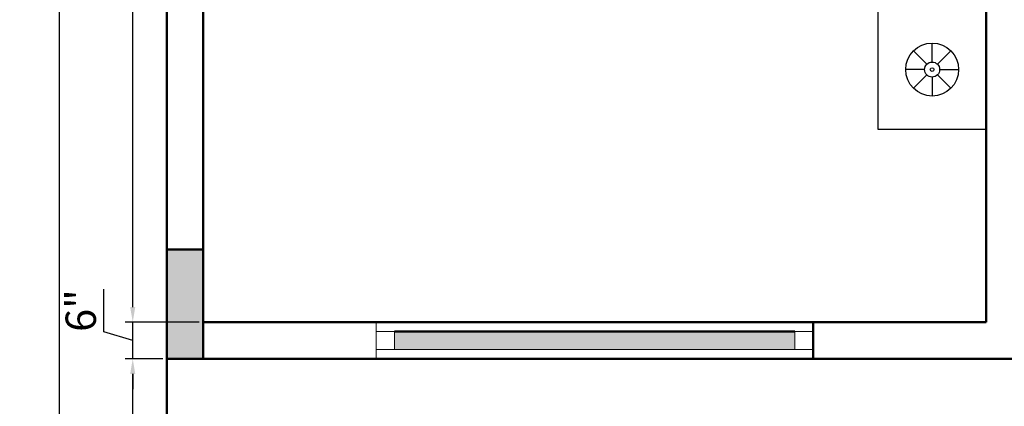
# Model space of a CAD drawing. Units: inches. Extents: x 3064 to 19385, y 846 to 15425.
# Tile 36 of 108: x 5167 to 5329, y 964 to 1028. Entities that reach past the tile are written whole.
import ezdxf

# ---------------------------------------------------------------- set-up
doc = ezdxf.new("R2010")
doc.units = ezdxf.units.IN
for name, color, linetype, lineweight in [('A-ANNO-DIMS', 2, 'Continuous', 18), ('A-COLS', 1, 'Continuous', 35), ('A-FLOR-FIXT', 9, 'Continuous', 18), ('A-GLAZ', 4, 'Continuous', 18), ('A-WALL', 7, 'Continuous', 50)]:
    doc.layers.add(name, color=color, linetype=linetype, lineweight=lineweight)
doc.layers.add('BLOCK', color=6, linetype='Continuous')
doc.styles.get("Standard").update_dxf_attribs({"font": 'arial.ttf'})
doc.dimstyles.new('ISO-25', dxfattribs={"dimtxt": 9, "dimasz": 2.5, "dimexe": 1.25, "dimexo": 0.625, "dimtad": 1, "dimdec": 1, "dimlunit": 3, "dimtxsty": 'Standard', "dimcen": 2.5, "dimadec": 0, "dimazin": 0, "dimtfac": 1, "dimtdec": 1, "dimtmove": 0, "dimatfit": 3, "dimfxl": 1, "dimarcsym": 0})

# ---------------------------------------------------------------- blocks, each defined once
blk = doc.blocks.new('A$C52E67D0D')
at = {"layer": 'BLOCK'}
for p, q in [((2229.3, 1596.3), (2173.3, 1652.3)), ((2251.5, 1605.5), (2251.5, 1684.7)), ((2273.7, 1596.3), (2329.7, 1652.3)), ((2220.1, 1574.1), (2140.9, 1574.1)), ((2282.9, 1574.1), (2362.1, 1574.1)), ((2229.3, 1551.9), (2173.3, 1495.9)), ((2251.5, 1542.8), (2251.5, 1463.5)), ((2273.7, 1551.9), (2329.7, 1495.9))]:
    blk.add_line(p, q, dxfattribs=at)
blk.add_lwpolyline([(2001, 1348.6), (2001, 1799.6), (2502, 1799.6), (2502, 1348.6)], close=True, dxfattribs=at)
for radius in [110.6, 31.4, 7.46]:
    blk.add_circle((2251.5, 1574.1), radius, dxfattribs=at)
blk = doc.blocks.new('*D68')
at = {"layer": 'A-ANNO-DIMS', "color": 0, "lineweight": -2, "transparency": 16777216}
for p, q in [((5190.39, 972.1), (5184.17, 972.1)), ((5185.42, 902.6), (5185.42, 969.6)), ((5190.39, 900.1), (5184.17, 900.1))]:
    blk.add_line(p, q, dxfattribs=at)
at = {"layer": 'A-ANNO-DIMS', "color": 0, "transparency": 16777216}
for points in [[(5185, 969.6), (5185.83, 969.6), (5185.42, 972.1)], [(5185, 902.6), (5185.83, 902.6), (5185.42, 900.1)]]:
    blk.add_solid(points, dxfattribs=at)
at = {"layer": 'Defpoints', "color": 0, "transparency": 16777216}
for p in [(5185.42, 972.1), (5191.02, 972.1), (5191.02, 900.1)]:
    blk.add_point(p, dxfattribs=at)
at = {"layer": 'A-ANNO-DIMS', "color": 0, "transparency": 16777216, "insert": (5182.24, 936.1), "char_height": 5, "attachment_point": 5, "rotation": 90}
blk.add_mtext("6'", dxfattribs=at)
blk = doc.blocks.new('*D69')
at = {"layer": 'A-ANNO-DIMS', "color": 0, "lineweight": -2, "transparency": 16777216}
for p, q in [((5180.68, 976.52), (5180.68, 983.54)), ((5185.42, 980.6), (5185.42, 983.1)), ((5196.39, 978.1), (5184.17, 978.1)), ((5185.42, 972.1), (5185.42, 978.1)), ((5185.42, 972.1), (5185.42, 978.1)), ((5185.42, 975.1), (5180.68, 976.52)), ((5190.39, 972.1), (5184.17, 972.1)), ((5185.42, 969.6), (5185.42, 967.1))]:
    blk.add_line(p, q, dxfattribs=at)
at = {"layer": 'A-ANNO-DIMS', "color": 0, "transparency": 16777216}
for points in [[(5185, 980.6), (5185.83, 980.6), (5185.42, 978.1)], [(5185, 969.6), (5185.83, 969.6), (5185.42, 972.1)]]:
    blk.add_solid(points, dxfattribs=at)
at = {"layer": 'Defpoints', "color": 0, "transparency": 16777216}
for p in [(5185.42, 978.1), (5197.02, 978.1), (5191.02, 972.1)]:
    blk.add_point(p, dxfattribs=at)
at = {"layer": 'A-ANNO-DIMS', "color": 0, "transparency": 16777216, "insert": (5177.5, 980.03), "char_height": 5, "attachment_point": 5, "rotation": 90}
blk.add_mtext('6"', dxfattribs=at)
blk = doc.blocks.new('*D70')
at = {"layer": 'A-ANNO-DIMS', "color": 0, "lineweight": -2, "transparency": 16777216}
for p, q in [((5196.39, 1176.1), (5184.17, 1176.1)), ((5185.42, 980.6), (5185.42, 1173.6)), ((5196.39, 978.1), (5184.17, 978.1))]:
    blk.add_line(p, q, dxfattribs=at)
at = {"layer": 'A-ANNO-DIMS', "color": 0, "transparency": 16777216}
for points in [[(5185, 1173.6), (5185.83, 1173.6), (5185.42, 1176.1)], [(5185, 980.6), (5185.83, 980.6), (5185.42, 978.1)]]:
    blk.add_solid(points, dxfattribs=at)
at = {"layer": 'Defpoints', "color": 0, "transparency": 16777216}
for p in [(5185.42, 1176.1), (5197.02, 1176.1), (5197.02, 978.1)]:
    blk.add_point(p, dxfattribs=at)
at = {"layer": 'A-ANNO-DIMS', "color": 0, "transparency": 16777216, "insert": (5182.24, 1077.1), "char_height": 5, "attachment_point": 5, "rotation": 90}
blk.add_mtext('16\'-6"', dxfattribs=at)
blk = doc.blocks.new('*D76')
at = {"layer": 'A-ANNO-DIMS', "color": 0, "lineweight": -2, "transparency": 16777216}
for p, q in [((5190.39, 1392.1), (5172.09, 1392.1)), ((5173.34, 902.6), (5173.34, 1389.6)), ((5190.39, 900.1), (5172.09, 900.1))]:
    blk.add_line(p, q, dxfattribs=at)
at = {"layer": 'A-ANNO-DIMS', "color": 0, "transparency": 16777216}
for points in [[(5172.92, 1389.6), (5173.75, 1389.6), (5173.34, 1392.1)], [(5172.92, 902.6), (5173.75, 902.6), (5173.34, 900.1)]]:
    blk.add_solid(points, dxfattribs=at)
at = {"layer": 'Defpoints', "color": 0, "transparency": 16777216}
for p in [(5173.34, 1392.1), (5191.02, 1392.1), (5191.02, 900.1)]:
    blk.add_point(p, dxfattribs=at)
at = {"layer": 'A-ANNO-DIMS', "color": 0, "transparency": 16777216, "insert": (5170.2, 1146.1), "char_height": 5, "attachment_point": 5, "rotation": 90}
blk.add_mtext("41'", dxfattribs=at)
blk = doc.blocks.new('WIN-1900')
blk.add_line((3, 0), (3, 66))
blk.add_lwpolyline([(3, 66), (0, 66), (0, 69), (3, 69)], close=True)

msp = doc.modelspace()

# ---------------------------------------------------------------- hatches: boundary and pattern name
at = {"layer": 'A-COLS'}
h = msp.add_hatch(color=256, dxfattribs=at)
h.dxf.hatch_style = 1
h.paths.add_polyline_path([(5197.02, 972.1), (5197.02, 990.1), (5191.02, 990.1), (5191.02, 972.1)])
at = {"layer": 'A-GLAZ'}
h = msp.add_hatch(color=256, dxfattribs=at)
h.dxf.hatch_style = 1
h.paths.add_polyline_path([(5228.52, 976.6), (5228.52, 973.6), (5294.52, 973.6), (5294.52, 976.6)])

# ---------------------------------------------------------------- linework, layer by layer
msp.add_line((5225.52, 972.1), (5225.52, 978.1), dxfattribs=at)
msp.add_lwpolyline([(5225.52, 973.6), (5225.52, 976.6), (5228.52, 976.6), (5228.52, 973.6)], close=True, dxfattribs=at)
at = {"layer": 'A-WALL'}
for p, q in [((5191.02, 1392.1), (5191.02, 972.1)), ((5197.02, 1176.1), (5197.02, 978.1)), ((5326.02, 1140.1), (5326.02, 978.1)), ((5326.02, 978.1), (5197.02, 978.1)), ((5228.52, 976.6), (5294.52, 976.6)), ((5297.52, 972.1), (5297.52, 978.1)), ((5533.02, 972.1), (5191.02, 972.1)), ((5197.02, 972.1), (5191.02, 972.1)), ((5191.02, 972.1), (5191.02, 900.1))]:
    msp.add_line(p, q, dxfattribs=at)
msp.add_lwpolyline([(5197.02, 972.1), (5197.02, 990.1), (5191.02, 990.1), (5191.02, 972.1)], close=True, dxfattribs=at)

# ---------------------------------------------------------------- block references
at = {"layer": 'A-FLOR-FIXT', "xscale": 0.039370099999992, "yscale": 0.039370099999992, "zscale": 0.039370099999992, "rotation": 270}
msp.add_blockref('A$C52E67D0D', (5255.15, 1108.35), dxfattribs=at)
at = {"layer": 'A-GLAZ', "rotation": 269.9999999999995}
msp.add_blockref('WIN-1900', (5228.52, 976.6), dxfattribs=at)

# ---------------------------------------------------------------- dimensions: what is measured, and where the dimension line sits
at = {"layer": 'A-ANNO-DIMS'}
for base, p1, p2, override, picture, middle in [((5173.34, 1392.1), (5191.02, 900.1), (5191.02, 1392.1), {"dimtxt": 5, "dimclrd": 0, "dimclre": 0, "dimclrt": 0}, '*D76', (5170.2, 1146.1)), ((5185.42, 1176.1), (5197.02, 978.1), (5197.02, 1176.1), {"dimtxt": 5, "dimclrd": 0, "dimclre": 0, "dimclrt": 0, "dimtmove": 1}, '*D70', (5182.24, 1077.1)), ((5185.42, 978.1), (5191.02, 972.1), (5197.02, 978.1), {"dimtxt": 5, "dimclrd": 0, "dimclre": 0, "dimclrt": 0, "dimtmove": 1}, '*D69', (5177.5, 977.14)), ((5185.42, 972.1), (5191.02, 900.1), (5191.02, 972.1), {"dimtxt": 5, "dimclrd": 0, "dimclre": 0, "dimclrt": 0}, '*D68', (5182.24, 936.1))]:
    dim = msp.add_linear_dim(base=base, p1=p1, p2=p2, angle=90, dimstyle='ISO-25', override=override, dxfattribs=at)
    dim.commit()
    dim.dimension.update_dxf_attribs({"geometry": picture, "text_midpoint": middle})

doc.saveas('drawing.dxf')
